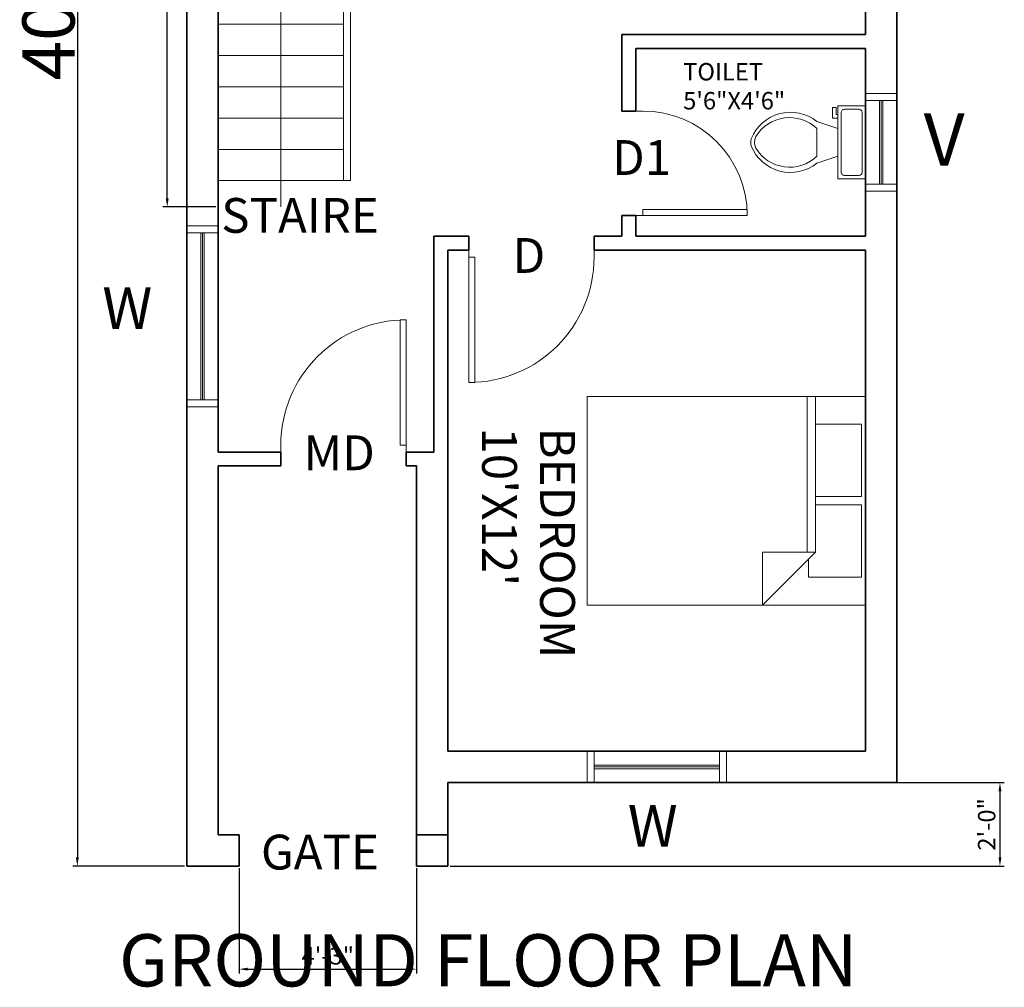
# Model space of a CAD drawing. Units: inches. Extents: x 1662 to 23131, y 1265 to 19127.
# Tile 14 of 26: x 19454 to 19737, y 8224 to 8502. Entities that reach past the tile are written whole.
import ezdxf

# ---------------------------------------------------------------- set-up
doc = ezdxf.new("R2010")
doc.units = ezdxf.units.IN
for name, color, linetype, lineweight in [('A-ANNO-DIMS', 4, 'Continuous', 18), ('A-ANNO-IDEN', 7, 'Continuous', 18), ('A-ANNO-TITL', 7, 'Continuous', 35), ('A-AREA-IDEN', 7, 'Continuous', 18), ('A-DOOR', 3, 'Continuous', 18), ('A-FLOR-FIXT', 9, 'Continuous', 18), ('A-FLOR-STRS', 7, 'Continuous', 18), ('A-FURN', 8, 'Continuous', 18), ('A-GLAZ', 4, 'Continuous', 18), ('A-WALL', 7, 'Continuous', 35)]:
    doc.layers.add(name, color=color, linetype=linetype, lineweight=lineweight)
doc.styles.get("Standard").update_dxf_attribs({"font": 'arial.ttf'})
doc.dimstyles.new('ISO-25', dxfattribs={"dimtxt": 5, "dimasz": 2.5, "dimexe": 1.25, "dimexo": 0.625, "dimtad": 1, "dimlunit": 3, "dimtxsty": 'Standard', "dimcen": 2.5, "dimadec": 0, "dimazin": 0, "dimtfac": 1, "dimtmove": 0, "dimatfit": 3, "dimfxl": 1, "dimarcsym": 0})

# ---------------------------------------------------------------- blocks, each defined once
blk = doc.blocks.new('Bed - Queen')
for p, q in [((0, -80.00003), (0, 0)), ((0, 0), (59.99999, 0)), ((59.99999, 0), (59.99999, -80.00003)), ((7.99999, -1.2), (28.79998, -1.2)), ((7.99999, -14.4), (7.99999, -1.2)), ((28.79998, -1.2), (28.79998, -14.4)), ((31.19999, -1.2), (51.99999, -1.2)), ((31.19999, -14.4), (31.19999, -1.2)), ((51.99999, -1.2), (51.99999, -16.4)), ((0, -14.4), (44.8, -14.4)), ((44.8, -16.8), (0, -16.8)), ((59.99999, -29.6), (44.8, -14.4)), ((44.8, -14.4), (44.8, -29.6)), ((51.99999, -16.4), (46.79936, -16.4)), ((44.8, -29.6), (59.99999, -29.6)), ((59.99999, -80.00003), (0, -80.00003))]:
    blk.add_line(p, q)
blk = doc.blocks.new('Toilet - top')
for p, q in [((9.5, -6), (9.5, -2)), ((-8, -8.5), (-8, -8)), ((-7, -8), (-7, -9.5)), ((-4, -8), (-6, -14)), ((4, -8), (6, -14)), ((-10, -8.5), (-8, -8.5)), ((-10, -9.5), (-10, -8.5)), ((-7, -9.5), (-10, -9.5)), ((4, -14), (-4, -14))]:
    blk.add_line(p, q)
blk.add_lwpolyline([(10.5, -8), (10.5, 0), (-10.5, 0), (-10.5, -8)], close=True)
for points in [[(-9.5, -2), (-9.5, -6)], [(8.5, -1), (-8.5, -1)], [(-8.5, -7), (8.5, -7)]]:
    blk.add_lwpolyline(points)
for centre, radius, start, end in [((-8.62, -1.88), 0.884, 81.8699, 188.1301), ((8.62, -1.88), 0.884, 351.8699, 98.1301), ((-8.62, -6.12), 0.884, 171.8699, 278.1301), ((8.62, -6.12), 0.884, 261.8699, 8.1301), ((3.52, -21.58), 12.17, 141.4691, 247.9714), ((4.2, -21.82), 11.33, 136.3677, 238.9468), ((-3.52, -21.58), 12.17, 292.0284, 38.5307), ((-4.2, -21.82), 11.33, 301.053, 43.6321), ((0, -27.88), 4, 245.7318, 294.2682), ((0, -29), 4, 254.8605, 285.1395)]:
    blk.add_arc(centre, radius, start, end)
blk = doc.blocks.new('*U88')
for p, q in [((0, 0), (0, 6)), ((36, 0), (36, 6))]:
    blk.add_line(p, q)
blk.add_lwpolyline([(0, 0), (0, -36), (1.75, -36), (1.75, 0)], close=True)
blk.add_arc((0, 0), 36, 270, 0)
blk = doc.blocks.new('*U89')
for p, q in [((-36, 0), (-36, -6)), ((0, 0), (0, -6))]:
    blk.add_line(p, q)
blk.add_lwpolyline([(0, 0), (0, 36), (-1.75, 36), (-1.75, 0)], close=True)
blk.add_arc((0, 0), 36, 90, 180)
blk = doc.blocks.new('*U93')
for p, q in [((-30, 0), (-30, -6)), ((0, 0), (0, -6))]:
    blk.add_line(p, q)
blk.add_lwpolyline([(0, 0), (0, 30), (-1.75, 30), (-1.75, 0)], close=True)
blk.add_arc((0, 0), 30, 90, 180)
blk = doc.blocks.new('*D95')
at = {"layer": 'A-ANNO-DIMS', "color": 0, "lineweight": -2, "transparency": 16777216}
for p, q in [((19501.54, 8738.72), (19469.46, 8738.72)), ((19470.71, 8736.22), (19470.71, 8261.22)), ((19501.54, 8258.72), (19469.46, 8258.72))]:
    blk.add_line(p, q, dxfattribs=at)
at = {"layer": 'A-ANNO-DIMS', "color": 0, "transparency": 16777216}
for points in [[(19470.29, 8736.22), (19471.12, 8736.22), (19470.71, 8738.72)], [(19470.29, 8261.22), (19471.12, 8261.22), (19470.71, 8258.72)]]:
    blk.add_solid(points, dxfattribs=at)
at = {"layer": 'Defpoints', "color": 0, "transparency": 16777216}
for p in [(19502.16, 8738.72), (19470.71, 8258.72), (19502.16, 8258.72)]:
    blk.add_point(p, dxfattribs=at)
at = {"layer": 'A-ANNO-DIMS', "color": 0, "transparency": 16777216, "insert": (19462.42, 8498.72), "char_height": 5, "attachment_point": 5, "rotation": 90}
blk.add_mtext("{\\H3x;40'}", dxfattribs=at)
blk = doc.blocks.new('WIN-48-J9X2')
for p, q in [((9, 52), (0, 52)), ((9, 50), (0, 50)), ((4, 50), (4, 2)), ((4.5, 50), (4.5, 2)), ((5, 50), (5, 2)), ((9, 2), (0, 2)), ((9, 0), (0, 0))]:
    blk.add_line(p, q)
blk = doc.blocks.new('VENT-24-J9X2')
for p, q in [((9, 28), (0, 28)), ((9, 26), (0, 26)), ((4, 26), (4, 2)), ((4.5, 26), (4.5, 2)), ((5, 26), (5, 2)), ((9, 2), (0, 2)), ((9, 0), (0, 0))]:
    blk.add_line(p, q)
blk = doc.blocks.new('WIN-36-J9X2')
for p, q in [((0, 0), (0, 9)), ((2, 0), (2, 9)), ((38, 0), (38, 9)), ((40, 0), (40, 9)), ((38, 5), (2, 5)), ((38, 4.5), (2, 4.5)), ((38, 4), (2, 4))]:
    blk.add_line(p, q)
blk = doc.blocks.new('STAIR-QUARTER-TURN')
for p, q in [((36, 61.57), (0, 97.57)), ((36, 61.57), (36, 97.57)), ((45, 61.57), (45, 97.57)), ((54, 61.57), (54, 97.57)), ((62, 59.57), (62, 97.57)), ((57.46, 79.57), (49.14, 86.54)), ((18, 79.57), (18, 0)), ((18, 79.57), (57.46, 79.57)), ((57.46, 79.57), (47.96, 73.62)), ((36, 61.57), (0, 61.57)), ((36, 7.57), (36, 61.57)), ((36, 61.57), (62, 61.57)), ((38, 7.57), (38, 59.57)), ((38, 59.57), (62, 59.57)), ((36, 52.57), (0, 52.57)), ((36, 43.57), (0, 43.57)), ((36, 34.57), (0, 34.57)), ((36, 25.57), (0, 25.57)), ((36, 16.57), (0, 16.57)), ((38, 7.57), (0, 7.57))]:
    blk.add_line(p, q)
blk = doc.blocks.new('*D193')
at = {"layer": 'A-ANNO-DIMS', "color": 0, "lineweight": -2, "transparency": 16777216}
for p, q in [((19496.53, 8545.72), (19496.53, 8671.92)), ((19510.54, 8545.72), (19495.28, 8545.72)), ((19496.53, 8450.65), (19496.53, 8543.22)), ((19510.54, 8448.15), (19495.28, 8448.15))]:
    blk.add_line(p, q, dxfattribs=at)
at = {"layer": 'A-ANNO-DIMS', "color": 0, "transparency": 16777216}
for points in [[(19496.11, 8543.22), (19496.94, 8543.22), (19496.53, 8545.72)], [(19496.11, 8450.65), (19496.94, 8450.65), (19496.53, 8448.15)]]:
    blk.add_solid(points, dxfattribs=at)
at = {"layer": 'Defpoints', "color": 0, "transparency": 16777216}
for p in [(19496.53, 8545.72), (19511.16, 8545.72), (19511.16, 8448.15)]:
    blk.add_point(p, dxfattribs=at)
at = {"layer": 'A-ANNO-DIMS', "color": 0, "transparency": 16777216, "insert": (19493.16, 8610.07), "char_height": 5, "attachment_point": 5, "rotation": 90}
blk.add_mtext('QUARTER-TURN STAIR 8\'-1 1/2" TYP.', dxfattribs=at)
blk = doc.blocks.new('*D241')
at = {"layer": 'A-ANNO-DIMS', "color": 0, "lineweight": -2, "transparency": 16777216}
for p, q in [((19517.16, 8258.1), (19517.16, 8227.87)), ((19568.16, 8258.1), (19568.16, 8227.87)), ((19519.66, 8229.12), (19565.66, 8229.12))]:
    blk.add_line(p, q, dxfattribs=at)
at = {"layer": 'A-ANNO-DIMS', "color": 0, "transparency": 16777216}
for points in [[(19519.66, 8229.54), (19519.66, 8228.71), (19517.16, 8229.12)], [(19565.66, 8229.54), (19565.66, 8228.71), (19568.16, 8229.12)]]:
    blk.add_solid(points, dxfattribs=at)
at = {"layer": 'Defpoints', "color": 0, "transparency": 16777216}
for p in [(19517.16, 8258.72), (19568.16, 8258.72), (19568.16, 8229.12)]:
    blk.add_point(p, dxfattribs=at)
at = {"layer": 'A-ANNO-DIMS', "color": 0, "transparency": 16777216, "insert": (19542.66, 8232.3), "char_height": 5, "attachment_point": 5}
blk.add_mtext('4\'-3"', dxfattribs=at)
blk = doc.blocks.new('*D242')
at = {"layer": 'A-ANNO-DIMS', "color": 0, "lineweight": -2, "transparency": 16777216}
for p, q in [((19577.79, 8282.72), (19737.01, 8282.72)), ((19735.76, 8280.22), (19735.76, 8261.22)), ((19577.79, 8258.72), (19737.01, 8258.72))]:
    blk.add_line(p, q, dxfattribs=at)
at = {"layer": 'A-ANNO-DIMS', "color": 0, "transparency": 16777216}
for points in [[(19735.35, 8280.22), (19736.18, 8280.22), (19735.76, 8282.72)], [(19735.35, 8261.22), (19736.18, 8261.22), (19735.76, 8258.72)]]:
    blk.add_solid(points, dxfattribs=at)
at = {"layer": 'Defpoints', "color": 0, "transparency": 16777216}
for p in [(19577.16, 8282.72), (19577.16, 8258.72), (19735.76, 8258.72)]:
    blk.add_point(p, dxfattribs=at)
at = {"layer": 'A-ANNO-DIMS', "color": 0, "transparency": 16777216, "insert": (19732.59, 8270.72), "char_height": 5, "attachment_point": 5, "rotation": 90}
blk.add_mtext('2\'-0"', dxfattribs=at)

msp = doc.modelspace()

# ---------------------------------------------------------------- linework, layer by layer
at = {"layer": 'A-WALL'}
for p, q in [((19502.163, 8258.722), (19502.163, 8738.722)), ((19706.163, 8738.722), (19706.163, 8282.722)), ((19697.163, 8639.722), (19697.163, 8497.722)), ((19511.163, 8377.722), (19511.163, 8545.722)), ((19697.163, 8497.722), (19627.163, 8497.722)), ((19627.163, 8497.722), (19627.163, 8475.722)), ((19697.163, 8493.722), (19631.163, 8493.722)), ((19631.163, 8493.722), (19631.163, 8475.722)), ((19697.163, 8493.722), (19697.163, 8439.722)), ((19631.163, 8475.722), (19627.163, 8475.722)), ((19631.163, 8445.722), (19627.163, 8445.722)), ((19627.163, 8445.722), (19627.163, 8439.722)), ((19631.163, 8445.722), (19631.163, 8439.722)), ((19573.163, 8439.722), (19573.163, 8377.722)), ((19583.163, 8439.722), (19573.163, 8439.722)), ((19583.163, 8439.722), (19583.163, 8435.722)), ((19627.163, 8439.722), (19619.163, 8439.722)), ((19619.163, 8439.722), (19619.163, 8435.722)), ((19697.163, 8439.722), (19631.163, 8439.722)), ((19577.163, 8435.722), (19577.163, 8291.722)), ((19583.163, 8435.722), (19577.163, 8435.722)), ((19697.163, 8435.722), (19619.163, 8435.722)), ((19697.163, 8435.722), (19697.163, 8291.722)), ((19511.163, 8377.722), (19529.163, 8377.722)), ((19529.163, 8373.722), (19529.163, 8377.722)), ((19565.163, 8377.722), (19573.163, 8377.722)), ((19565.163, 8373.722), (19565.163, 8377.722)), ((19511.163, 8267.722), (19511.163, 8373.722)), ((19511.163, 8373.722), (19529.163, 8373.722)), ((19565.163, 8373.722), (19568.163, 8373.722)), ((19568.163, 8373.722), (19568.163, 8258.722)), ((19577.163, 8373.722), (19577.163, 8291.722)), ((19697.163, 8291.722), (19577.163, 8291.722)), ((19706.163, 8282.722), (19577.163, 8282.722)), ((19577.163, 8282.722), (19577.163, 8258.722)), ((19517.163, 8267.722), (19511.163, 8267.722)), ((19517.163, 8267.722), (19517.163, 8258.722)), ((19577.163, 8267.722), (19568.163, 8267.722)), ((19517.163, 8258.722), (19502.163, 8258.722)), ((19577.163, 8258.722), (19568.163, 8258.722))]:
    msp.add_line(p, q, dxfattribs=at)

# ---------------------------------------------------------------- block references
at = {"layer": 'A-DOOR', "rotation": 270}
msp.add_blockref('*U93', (19633.163, 8445.722), dxfattribs=at)
at = {"layer": 'A-DOOR'}
for name, p in [('*U88', (19583.163, 8433.722)), ('*U89', (19565.163, 8379.722))]:
    msp.add_blockref(name, p, dxfattribs=at)
at = {"layer": 'A-FLOR-FIXT', "rotation": 270}
msp.add_blockref('Toilet - top', (19697.163, 8466.722), dxfattribs=at)
at = {"layer": 'A-FLOR-STRS'}
msp.add_blockref('STAIR-QUARTER-TURN', (19511.163, 8448.15), dxfattribs=at)
at = {"layer": 'A-FURN', "rotation": 270}
msp.add_blockref('Bed - Queen', (19697.163, 8393.722), dxfattribs=at)
at = {"layer": 'A-GLAZ'}
for name, p in [('VENT-24-J9X2', (19697.163, 8452.722)), ('WIN-48-J9X2', (19502.163, 8390.722)), ('WIN-36-J9X2', (19617.163, 8282.722))]:
    msp.add_blockref(name, p, dxfattribs=at)

# ---------------------------------------------------------------- texts
at = {"layer": 'A-ANNO-IDEN', "attachment_point": 1}
for s, width, heights, insert, char_height in [('V', 1142.59551, [20], (19713.85, 8475.064), 15), ('D1', 1142.59551, [20], (19624.322, 8467.366), 10), ('D', 1142.59551, [0], (19595.748, 8439.223), 10), ('W', 471.52273, [28.462], (19477.873, 8425.102), 12), ('MD', 1142.59551, [0], (19535.703, 8382.516), 10), ('W', 471.52273, [28.462], (19628.826, 8276.318), 12)]:
    msp.add_mtext_dynamic_manual_height_columns(s, width=width, gutter_width=12.5, heights=heights, dxfattribs=dict(at, insert=insert, char_height=char_height))
at = {"layer": 'A-ANNO-TITL', "insert": (19482.671, 8239.166), "char_height": 15, "attachment_point": 1}
msp.add_mtext_dynamic_manual_height_columns('GROUND FLOOR PLAN', width=1142.59551, gutter_width=12.5, heights=[0], dxfattribs=at)
at = {"layer": 'A-AREA-IDEN', "attachment_point": 1}
for s, heights, insert, char_height in [('TOILET\\P5\'6"X4\'6"', [277.772], (19644.748, 8489.527), 5), ('STAIRE', [0], (19512.048, 8450.729), 10), ('GATE', [0], (19523.463, 8267.758), 10)]:
    msp.add_mtext_dynamic_manual_height_columns(s, width=1142.59551, gutter_width=12.5, heights=heights, dxfattribs=dict(at, insert=insert, char_height=char_height))
at = {"layer": 'A-AREA-IDEN', "insert": (19613.664, 8384.809), "char_height": 10, "attachment_point": 1, "rotation": 270}
msp.add_mtext_dynamic_manual_height_columns("BEDROOM\\P10'X12'", width=1142.59551, gutter_width=12.5, heights=[277.772], dxfattribs=at)

# ---------------------------------------------------------------- dimensions: what is measured, and where the dimension line sits
at = {"layer": 'A-ANNO-DIMS'}
for base, p1, p2, text, override, picture, middle in [((19470.707, 8258.722), (19502.163, 8738.722), (19502.163, 8258.722), '{\\H3x;<>}', {"dimclrd": 0, "dimclre": 0, "dimclrt": 0}, '*D95', (19462.424, 8498.722)), ((19496.528, 8545.722), (19511.163, 8448.15), (19511.163, 8545.722), 'QUARTER-TURN STAIR <> TYP.', {"dimdec": 1, "dimlfac": 1, "dimrnd": 0, "dimzin": 1, "dimdsep": 46, "dimlunit": 4, "dimfrac": 2}, '*D193', (19493.164, 8610.07))]:
    dim = msp.add_linear_dim(base=base, p1=p1, p2=p2, angle=90, text=text, dimstyle='ISO-25', override=override, dxfattribs=at)
    dim.commit()
    dim.dimension.update_dxf_attribs({"geometry": picture, "text_midpoint": middle})
dim = msp.add_linear_dim(base=(19735.763, 8258.722), p1=(19577.163, 8282.722), p2=(19577.163, 8258.722), angle=90, dimstyle='ISO-25', override={"dimdec": 1, "dimlfac": 1, "dimrnd": 0, "dimzin": 1, "dimdsep": 46, "dimlunit": 4, "dimfrac": 2}, dxfattribs=at)
dim.commit()
dim.dimension.update_dxf_attribs({"geometry": '*D242', "text_midpoint": (19732.585, 8270.722)})
dim = msp.add_linear_dim(base=(19568.163, 8229.122), p1=(19517.163, 8258.722), p2=(19568.163, 8258.722), dimstyle='ISO-25', override={"dimdec": 1, "dimlfac": 1, "dimrnd": 0, "dimzin": 1, "dimdsep": 46, "dimlunit": 4, "dimfrac": 2}, dxfattribs=at)
dim.commit()
dim.dimension.update_dxf_attribs({"geometry": '*D241', "text_midpoint": (19542.663, 8232.302)})

doc.saveas('drawing.dxf')
